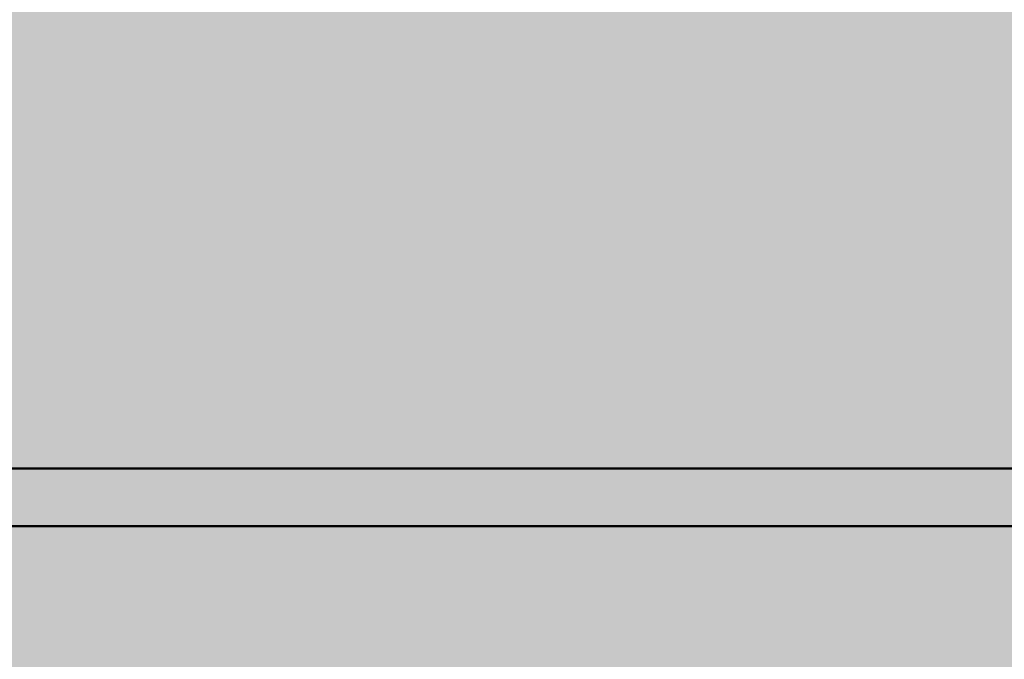
# Model space of a CAD drawing. Units: millimetres. Extents: x 0 to 2267, y 0 to 1823.
# Tile 136 of 256: x 1675 to 1760, y 1216 to 1271. Entities that reach past the tile are written whole.
import ezdxf

# ---------------------------------------------------------------- set-up
doc = ezdxf.new("R2010")
doc.units = ezdxf.units.MM
doc.header["$MEASUREMENT"] = 0
doc.layers.add('M-HATC', color=252, linetype='Continuous', lineweight=18)
doc.layers.add('M-OUTL', color=7, linetype='Continuous', lineweight=50)

msp = doc.modelspace()

# ---------------------------------------------------------------- hatches: boundary and pattern name
at = {"layer": 'M-HATC'}
h = msp.add_hatch(color=256, dxfattribs=at)
h.dxf.hatch_style = 1
h.paths.add_polyline_path([(2065.771, 1618.062, 0.236068), (2055.771, 1638.062), (1381.087, 1638.062, 0.236068), (1371.087, 1618.062), (1371.087, 1603.062), (2055.771, 1603.062), (2065.771, 1603.062)])
h.paths.add_polyline_path([(2062.772, 1550.296), (2062.772, 1560.296), (1374.086, 1560.296), (1374.086, 1550.296), (1374.086, 1540.296), (1384.086, 1540.296), (1389.086, 1540.296), (2062.772, 1540.296)])
h.paths.add_polyline_path([(1930.929, 1282.766), (1505.929, 1282.766), (1587.628, 1235.597, 0.131652), (1600.128, 1232.247), (1836.73, 1232.247, 0.131652), (1849.23, 1235.597)])
h.paths.add_polyline_path([(1930.929, 1117.417), (1905.929, 1117.417), (1505.929, 1117.417), (1505.929, 1077.417), (1930.929, 1077.417)])
h = msp.add_hatch(color=256, dxfattribs=at)
h.dxf.hatch_style = 1
h.paths.add_polyline_path([(2055.771, 1603.062), (1381.087, 1603.062), (1381.087, 1598.062), (2055.771, 1598.062)])
h.paths.add_polyline_path([(2055.771, 1598.062), (1381.087, 1598.062), (1381.087, 1593.062), (2055.771, 1593.062)])
h.paths.add_polyline_path([(2051.307, 1536.761), (1385.55, 1536.761), (1385.55, 1526.761), (1387.55, 1526.761), (1388.537, 1525.053), (1385.332, 1521.233), (1385.332, 1521.223), (2050.254, 1522.749), (2048.321, 1525.053), (2049.307, 1526.761), (2051.307, 1526.761)])
edge = h.paths.add_edge_path()
edge.add_arc((1847.535, 1379.149), 135, 222.60306, 222.89085, ccw=False)
edge.add_line((1748.166, 1287.766), (1683.092, 1287.766))
edge.add_arc((1583.724, 1379.149), 135, 317.10915, 317.39694, ccw=False)
edge.add_arc((1678.969, 1290.671), 5, 222.89085, 317.10915, ccw=False)
edge.add_arc((1774.213, 1379.149), 135, 222.60306, 222.89085, ccw=False)
edge.add_line((1674.845, 1287.766), (1609.771, 1287.766))
edge.add_arc((1510.403, 1379.149), 135, 317.10915, 317.39694, ccw=False)
edge.add_arc((1605.647, 1290.671), 5, 222.89085, 317.10915, ccw=False)
edge.add_arc((1700.892, 1379.149), 135, 222.60306, 222.89085, ccw=False)
edge.add_line((1601.524, 1287.766), (1536.45, 1287.766))
edge.add_arc((1437.081, 1379.149), 135, 317.10915, 317.39694, ccw=False)
edge.add_arc((1532.326, 1290.671), 5, 222.89085, 317.10915, ccw=False)
edge.add_arc((1627.571, 1379.149), 135, 222.60306, 222.89085, ccw=False)
edge.add_line((1528.203, 1287.766), (1505.929, 1287.766))
edge.add_spline(control_points=[(1505.929, 1287.766), (1504.262, 1287.766), (1504.262, 1282.766), (1505.929, 1282.766)], knot_values=[0, 0, 0, 0, 5, 5, 5, 5], degree=3, periodic=0)
edge.add_line((1505.929, 1282.766), (1930.929, 1282.766))
edge.add_spline(control_points=[(1930.929, 1282.766), (1932.596, 1282.766), (1932.596, 1287.766), (1930.929, 1287.766)], knot_values=[0, 0, 0, 0, 5, 5, 5, 5], degree=3, periodic=0)
edge.add_line((1930.929, 1287.766), (1903.056, 1287.766))
edge.add_arc((1803.688, 1379.149), 135, 317.10915, 317.39694, ccw=False)
edge.add_arc((1898.932, 1290.671), 5, 222.89085, 317.10915, ccw=False)
edge.add_arc((1994.177, 1379.149), 135, 222.60306, 222.89085, ccw=False)
edge.add_line((1894.809, 1287.766), (1829.735, 1287.766))
edge.add_arc((1730.366, 1379.149), 135, 317.10915, 317.39694, ccw=False)
edge.add_arc((1825.611, 1290.671), 5, 222.89085, 317.10915, ccw=False)
edge.add_arc((1920.856, 1379.149), 135, 222.60306, 222.89085, ccw=False)
edge.add_line((1821.487, 1287.766), (1756.413, 1287.766))
edge.add_arc((1657.045, 1379.149), 135, 317.10915, 317.39694, ccw=False)
edge.add_arc((1752.29, 1290.671), 5, 222.89085, 317.10915, ccw=False)
edge = h.paths.add_edge_path()
edge.add_spline(control_points=[(1843.429, 1227.247), (1845.096, 1227.247), (1845.096, 1232.247), (1843.429, 1232.247)], knot_values=[0, 0, 0, 0, 5, 5, 5, 5], degree=3, periodic=0)
edge.add_line((1843.429, 1232.247), (1593.429, 1232.247))
edge.add_spline(control_points=[(1593.429, 1232.247), (1591.762, 1232.247), (1591.762, 1227.247), (1593.429, 1227.247)], knot_values=[0, 0, 0, 0, 5, 5, 5, 5], degree=3, periodic=0)
edge.add_line((1593.429, 1227.247), (1843.429, 1227.247))
h.paths.add_polyline_path([(1905.929, 1127.417), (1530.929, 1127.417, 0.414214), (1520.929, 1117.417), (1530.929, 1117.417), (1915.929, 1117.417, 0.414214)])
edge = h.paths.add_edge_path()
edge.add_arc((1397.086, 1498.408), 12.73, 90.78215, 190.87871, ccw=False)
edge.add_line((1396.912, 1511.136), (1428.01, 1511.349))
edge.add_line((1428.01, 1511.349), (1433.01, 1511.349))
edge.add_line((1433.01, 1511.349), (1434.439, 1511.349))
edge.add_arc((1419.474, 1498.08), 20, 41.561, 74.08211)
edge.add_line((1424.959, 1517.314), (1399.935, 1517.256))
edge.add_spline(control_points=[(1399.931, 1517.256), (1399.884, 1517.213), (1399.833, 1517.169), (1399.777, 1517.124)], knot_values=[11.567499, 11.567499, 11.567499, 11.567499, 11.814249, 11.814249, 11.814249, 11.814249], degree=3, periodic=0)
edge.add_spline(control_points=[(1399.633, 1517.01), (1399.583, 1516.972), (1399.531, 1516.934), (1399.476, 1516.895)], knot_values=[11.167718, 11.167718, 11.167718, 11.167718, 11.365188, 11.365188, 11.365188, 11.365188], degree=3, periodic=0)
edge.add_spline(control_points=[(1399.34, 1516.8), (1399.151, 1516.672), (1398.938, 1516.538), (1398.704, 1516.399)], knot_values=[10.376405, 10.376405, 10.376405, 10.376405, 11.00994, 11.00994, 11.00994, 11.00994], degree=3, periodic=0)
edge.add_spline(control_points=[(1398.657, 1516.372), (1398.579, 1516.326), (1398.498, 1516.28), (1398.415, 1516.233)], knot_values=[10.125175, 10.125175, 10.125175, 10.125175, 10.334406, 10.334406, 10.334406, 10.334406], degree=3, periodic=0)
edge.add_spline(control_points=[(1398.264, 1516.149), (1398.196, 1516.111), (1398.126, 1516.073), (1398.055, 1516.035)], knot_values=[9.832246, 9.832246, 9.832246, 9.832246, 9.999658, 9.999658, 9.999658, 9.999658], degree=3, periodic=0)
edge.add_spline(control_points=[(1397.999, 1516.005), (1397.731, 1515.862), (1397.446, 1515.717), (1397.147, 1515.571)], knot_values=[9.161808, 9.161808, 9.161808, 9.161808, 9.787769, 9.787769, 9.787769, 9.787769], degree=3, periodic=0)
edge.add_spline(control_points=[(1397.147, 1515.571), (1396.842, 1515.423), (1396.522, 1515.274), (1396.191, 1515.126)], knot_values=[8.524455, 8.524455, 8.524455, 8.524455, 9.161808, 9.161808, 9.161808, 9.161808], degree=3, periodic=0)
edge.add_spline(control_points=[(1396.078, 1515.076), (1395.985, 1515.035), (1395.892, 1514.994), (1395.798, 1514.953)], knot_values=[8.275193, 8.275193, 8.275193, 8.275193, 8.451726, 8.451726, 8.451726, 8.451726], degree=3, periodic=0)
edge.add_spline(control_points=[(1395.602, 1514.869), (1395.5, 1514.826), (1395.397, 1514.782), (1395.293, 1514.739)], knot_values=[7.962917, 7.962917, 7.962917, 7.962917, 8.152764, 8.152764, 8.152764, 8.152764], degree=3, periodic=0)
edge.add_spline(control_points=[(1395.212, 1514.706), (1394.828, 1514.547), (1394.435, 1514.393), (1394.036, 1514.244)], knot_values=[7.21254, 7.21254, 7.21254, 7.21254, 7.913148, 7.913148, 7.913148, 7.913148], degree=3, periodic=0)
edge.add_spline(control_points=[(1394.036, 1514.244), (1393.708, 1514.121), (1393.375, 1514.003), (1393.043, 1513.889)], knot_values=[6.633733, 6.633733, 6.633733, 6.633733, 7.21254, 7.21254, 7.21254, 7.21254], degree=3, periodic=0)
edge.add_spline(control_points=[(1392.821, 1513.815), (1392.72, 1513.781), (1392.618, 1513.748), (1392.517, 1513.715)], knot_values=[6.328796, 6.328796, 6.328796, 6.328796, 6.505493, 6.505493, 6.505493, 6.505493], degree=3, periodic=0)
edge.add_spline(control_points=[(1392.517, 1513.715), (1392.319, 1513.652), (1392.121, 1513.59), (1391.924, 1513.531)], knot_values=[5.984605, 5.984605, 5.984605, 5.984605, 6.328796, 6.328796, 6.328796, 6.328796], degree=3, periodic=0)
edge.add_spline(control_points=[(1391.792, 1513.491), (1391.312, 1513.35), (1390.838, 1513.224), (1390.378, 1513.117)], knot_values=[5.066697, 5.066697, 5.066697, 5.066697, 5.907055, 5.907055, 5.907055, 5.907055], degree=3, periodic=0)
edge.add_spline(control_points=[(1390.378, 1513.117), (1390.18, 1513.071), (1389.984, 1513.028), (1389.791, 1512.99)], knot_values=[4.70367, 4.70367, 4.70367, 4.70367, 5.066695, 5.066695, 5.066695, 5.066695], degree=3, periodic=0)
edge.add_spline(control_points=[(1389.422, 1512.92), (1389.246, 1512.889), (1389.073, 1512.862), (1388.904, 1512.838)], knot_values=[4.130571, 4.130571, 4.130571, 4.130571, 4.469816, 4.469816, 4.469816, 4.469816], degree=3, periodic=0)
edge.add_spline(control_points=[(1388.904, 1512.838), (1388.591, 1512.795), (1388.291, 1512.764), (1388.007, 1512.749)], knot_values=[3.504031, 3.504031, 3.504031, 3.504031, 4.130571, 4.130571, 4.130571, 4.130571], degree=3, periodic=0)
edge.add_spline(control_points=[(1387.936, 1512.746), (1387.854, 1512.742), (1387.773, 1512.74), (1387.694, 1512.739)], knot_values=[3.268866, 3.268866, 3.268866, 3.268866, 3.451164, 3.451164, 3.451164, 3.451164], degree=3, periodic=0)
edge.add_spline(control_points=[(1387.335, 1512.744), (1387.208, 1512.75), (1387.085, 1512.76), (1386.967, 1512.774)], knot_values=[2.670686, 2.670686, 2.670686, 2.670686, 2.984, 2.984, 2.984, 2.984], degree=3, periodic=0)
edge.add_spline(control_points=[(1386.833, 1512.792), (1386.821, 1512.794), (1386.809, 1512.796), (1386.797, 1512.798)], knot_values=[2.516981, 2.516981, 2.516981, 2.516981, 2.549528, 2.549528, 2.549528, 2.549528], degree=3, periodic=0)
edge.add_spline(control_points=[(1386.453, 1512.873), (1386.426, 1512.881), (1386.399, 1512.889), (1386.373, 1512.897)], knot_values=[2.095869, 2.095869, 2.095869, 2.095869, 2.17941, 2.17941, 2.17941, 2.17941], degree=3, periodic=0)
edge.add_spline(control_points=[(1386.069, 1513.019), (1386.063, 1513.022), (1386.058, 1513.025), (1386.052, 1513.028)], knot_values=[1.72453, 1.72453, 1.72453, 1.72453, 1.745933, 1.745933, 1.745933, 1.745933], degree=3, periodic=0)
edge.add_arc((1399.474, 1498.08), 20, 131.82432, 180)
edge.add_arc((1630.334, 1505.548), 250.971, 181.70518, 236.42798)
edge.add_arc((1605.34, 1483.304), 218.782, 238.66083, 243.34961)
edge.add_arc((1647.091, 1510.359), 262.899, 183.12984, 237.85344, ccw=False)
h.paths.add_polyline_path([(1406.537, 1391.964, 0.149382), (1491.551, 1296.442, -0.129517)], flags=17)
edge = h.paths.add_edge_path()
edge.add_arc((2037.384, 1498.08), 20, 0, 48.26587)
edge.add_spline(control_points=[(2050.697, 1513.005), (2050.651, 1512.985), (2050.603, 1512.966), (2050.554, 1512.948)], knot_values=[1.835652, 1.835652, 1.835652, 1.835652, 2.000781, 2.000781, 2.000781, 2.000781], degree=3, periodic=0)
edge.add_spline(control_points=[(2050.462, 1512.917), (2050.479, 1512.922), (2050.496, 1512.928), (2050.513, 1512.934)], knot_values=[2.045477, 2.045477, 2.045477, 2.045477, 2.101389, 2.101389, 2.101389, 2.101389], degree=3, periodic=0)
edge.add_spline(control_points=[(2050.129, 1512.834), (2050.198, 1512.847), (2050.266, 1512.862), (2050.331, 1512.879)], knot_values=[2.237629, 2.237629, 2.237629, 2.237629, 2.435841, 2.435841, 2.435841, 2.435841], degree=3, periodic=0)
edge.add_spline(control_points=[(2050.095, 1512.828), (2050.106, 1512.83), (2050.118, 1512.832), (2050.129, 1512.834)], knot_values=[2.435841, 2.435841, 2.435841, 2.435841, 2.468321, 2.468321, 2.468321, 2.468321], degree=3, periodic=0)
edge.add_spline(control_points=[(2049.784, 1512.785), (2049.855, 1512.792), (2049.924, 1512.801), (2049.992, 1512.811)], knot_values=[2.563852, 2.563852, 2.563852, 2.563852, 2.748541, 2.748541, 2.748541, 2.748541], degree=3, periodic=0)
edge.add_spline(control_points=[(2049.405, 1512.762), (2049.536, 1512.765), (2049.663, 1512.773), (2049.784, 1512.785)], knot_values=[2.748541, 2.748541, 2.748541, 2.748541, 3.064882, 3.064882, 3.064882, 3.064882], degree=3, periodic=0)
edge.add_spline(control_points=[(2049.17, 1512.76), (2049.234, 1512.759), (2049.297, 1512.759), (2049.358, 1512.761)], knot_values=[3.102309, 3.102309, 3.102309, 3.102309, 3.2503, 3.2503, 3.2503, 3.2503], degree=3, periodic=0)
edge.add_spline(control_points=[(2048.857, 1512.769), (2048.964, 1512.764), (2049.068, 1512.761), (2049.17, 1512.76)], knot_values=[3.2503, 3.2503, 3.2503, 3.2503, 3.486069, 3.486069, 3.486069, 3.486069], degree=3, periodic=0)
edge.add_spline(control_points=[(2048.692, 1512.779), (2048.373, 1512.801), (2048.035, 1512.841), (2047.682, 1512.897)], knot_values=[3.606429, 3.606429, 3.606429, 3.606429, 4.2989, 4.2989, 4.2989, 4.2989], degree=3, periodic=0)
edge.add_spline(control_points=[(2047.682, 1512.897), (2047.546, 1512.919), (2047.408, 1512.942), (2047.268, 1512.969)], knot_values=[4.2989, 4.2989, 4.2989, 4.2989, 4.565769, 4.565769, 4.565769, 4.565769], degree=3, periodic=0)
edge.add_spline(control_points=[(2047.268, 1512.969), (2047.145, 1512.991), (2047.021, 1513.016), (2046.895, 1513.042)], knot_values=[4.565769, 4.565769, 4.565769, 4.565769, 4.799971, 4.799971, 4.799971, 4.799971], degree=3, periodic=0)
edge.add_spline(control_points=[(2046.895, 1513.042), (2046.529, 1513.119), (2046.151, 1513.209), (2045.768, 1513.311)], knot_values=[4.799971, 4.799971, 4.799971, 4.799971, 5.483718, 5.483718, 5.483718, 5.483718], degree=3, periodic=0)
edge.add_spline(control_points=[(2045.768, 1513.311), (2045.372, 1513.415), (2044.97, 1513.532), (2044.566, 1513.659)], knot_values=[5.483718, 5.483718, 5.483718, 5.483718, 6.187866, 6.187866, 6.187866, 6.187866], degree=3, periodic=0)
edge.add_spline(control_points=[(2044.566, 1513.659), (2044.415, 1513.706), (2044.263, 1513.755), (2044.112, 1513.805)], knot_values=[6.187866, 6.187866, 6.187866, 6.187866, 6.451551, 6.451551, 6.451551, 6.451551], degree=3, periodic=0)
edge.add_spline(control_points=[(2044.112, 1513.805), (2043.997, 1513.843), (2043.882, 1513.881), (2043.767, 1513.92)], knot_values=[6.451551, 6.451551, 6.451551, 6.451551, 6.651434, 6.651434, 6.651434, 6.651434], degree=3, periodic=0)
edge.add_spline(control_points=[(2043.767, 1513.92), (2043.372, 1514.055), (2042.977, 1514.198), (2042.589, 1514.346)], knot_values=[6.651434, 6.651434, 6.651434, 6.651434, 7.338879, 7.338879, 7.338879, 7.338879], degree=3, periodic=0)
edge.add_spline(control_points=[(2042.589, 1514.346), (2042.164, 1514.507), (2041.746, 1514.675), (2041.341, 1514.846)], knot_values=[7.338879, 7.338879, 7.338879, 7.338879, 8.089209, 8.089209, 8.089209, 8.089209], degree=3, periodic=0)
edge.add_spline(control_points=[(2041.341, 1514.846), (2041.103, 1514.946), (2040.869, 1515.048), (2040.64, 1515.15)], knot_values=[8.089209, 8.089209, 8.089209, 8.089209, 8.529587, 8.529587, 8.529587, 8.529587], degree=3, periodic=0)
edge.add_spline(control_points=[(2040.51, 1515.209), (2040.082, 1515.402), (2039.675, 1515.597), (2039.295, 1515.789)], knot_values=[8.613818, 8.613818, 8.613818, 8.613818, 9.44571, 9.44571, 9.44571, 9.44571], degree=3, periodic=0)
edge.add_spline(control_points=[(2039.295, 1515.789), (2039.062, 1515.907), (2038.839, 1516.025), (2038.629, 1516.14)], knot_values=[9.44571, 9.44571, 9.44571, 9.44571, 9.956404, 9.956404, 9.956404, 9.956404], degree=3, periodic=0)
edge.add_spline(control_points=[(2038.629, 1516.14), (2038.519, 1516.2), (2038.412, 1516.26), (2038.309, 1516.319)], knot_values=[9.956404, 9.956404, 9.956404, 9.956404, 10.223542, 10.223542, 10.223542, 10.223542], degree=3, periodic=0)
edge.add_spline(control_points=[(2038.309, 1516.319), (2038.214, 1516.374), (2038.122, 1516.428), (2038.033, 1516.481)], knot_values=[10.223542, 10.223542, 10.223542, 10.223542, 10.47051, 10.47051, 10.47051, 10.47051], degree=3, periodic=0)
edge.add_spline(control_points=[(2038.033, 1516.481), (2037.786, 1516.63), (2037.564, 1516.773), (2037.372, 1516.909)], knot_values=[10.47051, 10.47051, 10.47051, 10.47051, 11.15767, 11.15767, 11.15767, 11.15767], degree=3, periodic=0)
edge.add_spline(control_points=[(2037.372, 1516.909), (2037.279, 1516.975), (2037.193, 1517.04), (2037.114, 1517.102)], knot_values=[11.15767, 11.15767, 11.15767, 11.15767, 11.49227, 11.49227, 11.49227, 11.49227], degree=3, periodic=0)
edge.add_spline(control_points=[(2036.856, 1517.326), (2036.915, 1517.269), (2036.981, 1517.21), (2037.056, 1517.149)], knot_values=[11.577341, 11.577341, 11.577341, 11.577341, 11.91035, 11.91035, 11.91035, 11.91035], degree=3, periodic=0)
edge.add_spline(control_points=[(2036.807, 1517.375), (2036.823, 1517.359), (2036.839, 1517.342), (2036.856, 1517.326)], knot_values=[11.91035, 11.91035, 11.91035, 11.91035, 12.007402, 12.007402, 12.007402, 12.007402], degree=3, periodic=0)
edge.add_spline(control_points=[(2036.702, 1517.494), (2036.71, 1517.483), (2036.72, 1517.472), (2036.729, 1517.461)], knot_values=[12.184155, 12.184155, 12.184155, 12.184155, 12.255409, 12.255409, 12.255409, 12.255409], degree=3, periodic=0)
edge.add_spline(control_points=[(2036.616, 1517.621), (2036.62, 1517.613), (2036.624, 1517.606), (2036.629, 1517.598)], knot_values=[12.487913, 12.487913, 12.487913, 12.487913, 12.541035, 12.541035, 12.541035, 12.541035], degree=3, periodic=0)
edge.add_spline(control_points=[(2036.563, 1517.786), (2036.564, 1517.779), (2036.564, 1517.773), (2036.565, 1517.766)], knot_values=[12.911761, 12.911761, 12.911761, 12.911761, 12.968286, 12.968286, 12.968286, 12.968286], degree=3, periodic=0)
edge.add_spline(control_points=[(2036.617, 1517.93), (2036.612, 1517.926), (2036.609, 1517.921), (2036.605, 1517.916)], knot_values=[13.382527, 13.382527, 13.382527, 13.382527, 13.433791, 13.433791, 13.433791, 13.433791], degree=3, periodic=0)
edge.add_spline(control_points=[(2036.749, 1518.017), (2036.736, 1518.012), (2036.724, 1518.006), (2036.712, 1518)], knot_values=[13.726299, 13.726299, 13.726299, 13.726299, 13.809928, 13.809928, 13.809928, 13.809928], degree=3, periodic=0)
edge.add_spline(control_points=[(2036.86, 1518.053), (2036.839, 1518.047), (2036.818, 1518.042), (2036.799, 1518.035)], knot_values=[13.910887, 13.910887, 13.910887, 13.910887, 14.02153, 14.02153, 14.02153, 14.02153], degree=3, periodic=0)
edge.add_line((2036.964, 1518.08), (2032.384, 1518.08))
edge.add_line((2032.384, 1518.08), (2027.384, 1518.08))
edge.add_line((2027.384, 1518.08), (2022.384, 1518.08))
edge.add_line((2022.384, 1518.08), (2017.384, 1518.08))
edge.add_arc((2017.384, 1498.08), 20, 90, 138.439)
edge.add_line((2002.419, 1511.349), (2003.848, 1511.349))
edge.add_line((2003.848, 1511.349), (2008.848, 1511.349))
edge.add_line((2008.848, 1511.349), (2039.772, 1511.138))
edge.add_arc((2039.772, 1498.408), 12.73, -10.87871, 90, ccw=False)
edge.add_arc((1789.767, 1510.359), 262.899, 302.14656, 356.87016, ccw=False)
edge.add_arc((1831.518, 1483.304), 218.782, 296.65039, 301.33917)
edge.add_arc((1806.524, 1505.548), 250.971, 303.57202, 358.29482)
h.paths.add_polyline_path([(2030.321, 1391.964, -0.129517), (1945.307, 1296.442, 0.149382)], flags=17)
edge = h.paths.add_edge_path()
edge.add_spline(control_points=[(2037.246, 1518.082), (2037.29, 1518.081), (2037.336, 1518.08), (2037.384, 1518.08)], knot_values=[0.000012, 0.000012, 0.000012, 0.000012, 0.144754, 0.144754, 0.144754, 0.144754], degree=3, periodic=0)
edge.add_line((2037.336, 1518.08), (2037.01, 1518.08))
edge.add_spline(control_points=[(2037.01, 1518.08), (2036.982, 1518.077), (2036.956, 1518.073), (2036.931, 1518.068)], knot_values=[14.13465, 14.13465, 14.13465, 14.13465, 14.247197, 14.247197, 14.247197, 14.247197], degree=3, periodic=0)
edge.add_spline(control_points=[(2036.931, 1518.068), (2036.928, 1518.067), (2036.924, 1518.067), (2036.921, 1518.066)], knot_values=[14.118315, 14.118315, 14.118315, 14.118315, 14.13465, 14.13465, 14.13465, 14.13465], degree=3, periodic=0)
edge.add_spline(control_points=[(2036.921, 1518.066), (2036.912, 1518.064), (2036.903, 1518.063), (2036.895, 1518.061)], knot_values=[14.078086, 14.078086, 14.078086, 14.078086, 14.118315, 14.118315, 14.118315, 14.118315], degree=3, periodic=0)
edge.add_spline(control_points=[(2036.895, 1518.061), (2036.883, 1518.058), (2036.872, 1518.056), (2036.86, 1518.053)], knot_values=[14.02153, 14.02153, 14.02153, 14.02153, 14.078086, 14.078086, 14.078086, 14.078086], degree=3, periodic=0)
edge.add_spline(control_points=[(2036.86, 1518.053), (2036.839, 1518.047), (2036.818, 1518.042), (2036.799, 1518.035)], knot_values=[13.910887, 13.910887, 13.910887, 13.910887, 14.02153, 14.02153, 14.02153, 14.02153], degree=3, periodic=0)
edge.add_spline(control_points=[(2036.799, 1518.035), (2036.798, 1518.035), (2036.797, 1518.035), (2036.797, 1518.035)], knot_values=[13.906906, 13.906906, 13.906906, 13.906906, 13.910887, 13.910887, 13.910887, 13.910887], degree=3, periodic=0)
edge.add_spline(control_points=[(2036.797, 1518.035), (2036.788, 1518.032), (2036.78, 1518.029), (2036.772, 1518.026)], knot_values=[13.857826, 13.857826, 13.857826, 13.857826, 13.906906, 13.906906, 13.906906, 13.906906], degree=3, periodic=0)
edge.add_spline(control_points=[(2036.772, 1518.026), (2036.764, 1518.023), (2036.756, 1518.02), (2036.749, 1518.017)], knot_values=[13.809928, 13.809928, 13.809928, 13.809928, 13.857826, 13.857826, 13.857826, 13.857826], degree=3, periodic=0)
edge.add_spline(control_points=[(2036.749, 1518.017), (2036.736, 1518.012), (2036.724, 1518.006), (2036.712, 1518)], knot_values=[13.726299, 13.726299, 13.726299, 13.726299, 13.809928, 13.809928, 13.809928, 13.809928], degree=3, periodic=0)
edge.add_spline(control_points=[(2036.712, 1518), (2036.712, 1518), (2036.712, 1518), (2036.711, 1518)], knot_values=[13.723993, 13.723993, 13.723993, 13.723993, 13.726299, 13.726299, 13.726299, 13.726299], degree=3, periodic=0)
edge.add_spline(control_points=[(2036.711, 1518), (2036.706, 1517.997), (2036.701, 1517.994), (2036.696, 1517.992)], knot_values=[13.686536, 13.686536, 13.686536, 13.686536, 13.723993, 13.723993, 13.723993, 13.723993], degree=3, periodic=0)
edge.add_spline(control_points=[(2036.696, 1517.992), (2036.692, 1517.989), (2036.687, 1517.987), (2036.683, 1517.984)], knot_values=[13.651251, 13.651251, 13.651251, 13.651251, 13.686536, 13.686536, 13.686536, 13.686536], degree=3, periodic=0)
edge.add_spline(control_points=[(2036.683, 1517.984), (2036.676, 1517.98), (2036.67, 1517.976), (2036.664, 1517.971)], knot_values=[13.596804, 13.596804, 13.596804, 13.596804, 13.651251, 13.651251, 13.651251, 13.651251], degree=3, periodic=0)
edge.add_spline(control_points=[(2036.664, 1517.971), (2036.664, 1517.971), (2036.663, 1517.971), (2036.663, 1517.971)], knot_values=[13.593956, 13.593956, 13.593956, 13.593956, 13.596804, 13.596804, 13.596804, 13.596804], degree=3, periodic=0)
edge.add_spline(control_points=[(2036.663, 1517.971), (2036.66, 1517.969), (2036.658, 1517.967), (2036.655, 1517.965)], knot_values=[13.570322, 13.570322, 13.570322, 13.570322, 13.593956, 13.593956, 13.593956, 13.593956], degree=3, periodic=0)
edge.add_spline(control_points=[(2036.655, 1517.965), (2036.653, 1517.963), (2036.65, 1517.961), (2036.647, 1517.959)], knot_values=[13.545477, 13.545477, 13.545477, 13.545477, 13.570322, 13.570322, 13.570322, 13.570322], degree=3, periodic=0)
edge.add_spline(control_points=[(2036.647, 1517.959), (2036.647, 1517.959), (2036.647, 1517.959), (2036.647, 1517.959)], knot_values=[13.543931, 13.543931, 13.543931, 13.543931, 13.545477, 13.545477, 13.545477, 13.545477], degree=3, periodic=0)
edge.add_spline(control_points=[(2036.647, 1517.959), (2036.641, 1517.954), (2036.636, 1517.949), (2036.631, 1517.945)], knot_values=[13.488237, 13.488237, 13.488237, 13.488237, 13.543931, 13.543931, 13.543931, 13.543931], degree=3, periodic=0)
edge.add_spline(control_points=[(2036.631, 1517.945), (2036.628, 1517.942), (2036.626, 1517.94), (2036.623, 1517.937)], knot_values=[13.460307, 13.460307, 13.460307, 13.460307, 13.488237, 13.488237, 13.488237, 13.488237], degree=3, periodic=0)
edge.add_spline(control_points=[(2036.623, 1517.937), (2036.622, 1517.936), (2036.62, 1517.934), (2036.618, 1517.932)], knot_values=[13.439712, 13.439712, 13.439712, 13.439712, 13.460307, 13.460307, 13.460307, 13.460307], degree=3, periodic=0)
edge.add_spline(control_points=[(2036.618, 1517.932), (2036.618, 1517.931), (2036.617, 1517.931), (2036.617, 1517.93)], knot_values=[13.433791, 13.433791, 13.433791, 13.433791, 13.439712, 13.439712, 13.439712, 13.439712], degree=3, periodic=0)
edge.add_spline(control_points=[(2036.617, 1517.93), (2036.612, 1517.926), (2036.609, 1517.921), (2036.605, 1517.916)], knot_values=[13.382527, 13.382527, 13.382527, 13.382527, 13.433791, 13.433791, 13.433791, 13.433791], degree=3, periodic=0)
edge.add_spline(control_points=[(2036.605, 1517.916), (2036.603, 1517.913), (2036.6, 1517.91), (2036.598, 1517.907)], knot_values=[13.350017, 13.350017, 13.350017, 13.350017, 13.382527, 13.382527, 13.382527, 13.382527], degree=3, periodic=0)
edge.add_spline(control_points=[(2036.598, 1517.907), (2036.597, 1517.906), (2036.596, 1517.904), (2036.595, 1517.903)], knot_values=[13.333922, 13.333922, 13.333922, 13.333922, 13.350017, 13.350017, 13.350017, 13.350017], degree=3, periodic=0)
edge.add_spline(control_points=[(2036.595, 1517.903), (2036.595, 1517.902), (2036.594, 1517.901), (2036.593, 1517.9)], knot_values=[13.323828, 13.323828, 13.323828, 13.323828, 13.333922, 13.333922, 13.333922, 13.333922], degree=3, periodic=0)
edge.add_spline(control_points=[(2036.593, 1517.9), (2036.59, 1517.895), (2036.588, 1517.891), (2036.585, 1517.886)], knot_values=[13.277545, 13.277545, 13.277545, 13.277545, 13.323828, 13.323828, 13.323828, 13.323828], degree=3, periodic=0)
edge.add_spline(control_points=[(2036.585, 1517.886), (2036.584, 1517.883), (2036.582, 1517.879), (2036.58, 1517.875)], knot_values=[13.240119, 13.240119, 13.240119, 13.240119, 13.277545, 13.277545, 13.277545, 13.277545], degree=3, periodic=0)
edge.add_spline(control_points=[(2036.58, 1517.875), (2036.58, 1517.874), (2036.579, 1517.873), (2036.578, 1517.872)], knot_values=[13.228211, 13.228211, 13.228211, 13.228211, 13.240119, 13.240119, 13.240119, 13.240119], degree=3, periodic=0)
edge.add_spline(control_points=[(2036.578, 1517.872), (2036.578, 1517.87), (2036.577, 1517.869), (2036.577, 1517.868)], knot_values=[13.215717, 13.215717, 13.215717, 13.215717, 13.228211, 13.228211, 13.228211, 13.228211], degree=3, periodic=0)
edge.add_spline(control_points=[(2036.577, 1517.868), (2036.575, 1517.864), (2036.574, 1517.86), (2036.573, 1517.857)], knot_values=[13.179847, 13.179847, 13.179847, 13.179847, 13.215717, 13.215717, 13.215717, 13.215717], degree=3, periodic=0)
edge.add_spline(control_points=[(2036.573, 1517.857), (2036.571, 1517.851), (2036.57, 1517.846), (2036.569, 1517.841)], knot_values=[13.132017, 13.132017, 13.132017, 13.132017, 13.179847, 13.179847, 13.179847, 13.179847], degree=3, periodic=0)
edge.add_spline(control_points=[(2036.569, 1517.841), (2036.568, 1517.84), (2036.568, 1517.839), (2036.568, 1517.838)], knot_values=[13.122482, 13.122482, 13.122482, 13.122482, 13.132017, 13.132017, 13.132017, 13.132017], degree=3, periodic=0)
edge.add_spline(control_points=[(2036.568, 1517.838), (2036.568, 1517.836), (2036.567, 1517.835), (2036.567, 1517.833)], knot_values=[13.105592, 13.105592, 13.105592, 13.105592, 13.122482, 13.122482, 13.122482, 13.122482], degree=3, periodic=0)
edge.add_spline(control_points=[(2036.567, 1517.833), (2036.566, 1517.829), (2036.566, 1517.826), (2036.565, 1517.822)], knot_values=[13.074063, 13.074063, 13.074063, 13.074063, 13.105592, 13.105592, 13.105592, 13.105592], degree=3, periodic=0)
edge.add_spline(control_points=[(2036.565, 1517.822), (2036.565, 1517.822), (2036.565, 1517.822), (2036.565, 1517.822)], knot_values=[13.074043, 13.074043, 13.074043, 13.074043, 13.074063, 13.074063, 13.074063, 13.074063], degree=3, periodic=0)
edge.add_spline(control_points=[(2036.565, 1517.822), (2036.564, 1517.816), (2036.564, 1517.811), (2036.564, 1517.805)], knot_values=[13.021884, 13.021884, 13.021884, 13.021884, 13.074043, 13.074043, 13.074043, 13.074043], degree=3, periodic=0)
edge.add_spline(control_points=[(2036.564, 1517.805), (2036.564, 1517.804), (2036.564, 1517.803), (2036.564, 1517.803)], knot_values=[13.01674, 13.01674, 13.01674, 13.01674, 13.021884, 13.021884, 13.021884, 13.021884], degree=3, periodic=0)
edge.add_spline(control_points=[(2036.564, 1517.803), (2036.563, 1517.801), (2036.563, 1517.798), (2036.563, 1517.796)], knot_values=[12.996438, 12.996438, 12.996438, 12.996438, 13.01674, 13.01674, 13.01674, 13.01674], degree=3, periodic=0)
edge.add_spline(control_points=[(2036.563, 1517.796), (2036.563, 1517.793), (2036.563, 1517.789), (2036.563, 1517.786)], knot_values=[12.968286, 12.968286, 12.968286, 12.968286, 12.996438, 12.996438, 12.996438, 12.996438], degree=3, periodic=0)
edge.add_spline(control_points=[(2036.563, 1517.786), (2036.564, 1517.779), (2036.564, 1517.773), (2036.565, 1517.766)], knot_values=[12.911761, 12.911761, 12.911761, 12.911761, 12.968286, 12.968286, 12.968286, 12.968286], degree=3, periodic=0)
edge.add_spline(control_points=[(2036.565, 1517.766), (2036.565, 1517.766), (2036.565, 1517.766), (2036.565, 1517.766)], knot_values=[12.911017, 12.911017, 12.911017, 12.911017, 12.911761, 12.911761, 12.911761, 12.911761], degree=3, periodic=0)
edge.add_spline(control_points=[(2036.565, 1517.766), (2036.565, 1517.762), (2036.566, 1517.759), (2036.566, 1517.756)], knot_values=[12.88528, 12.88528, 12.88528, 12.88528, 12.911017, 12.911017, 12.911017, 12.911017], degree=3, periodic=0)
edge.add_spline(control_points=[(2036.566, 1517.756), (2036.567, 1517.753), (2036.567, 1517.751), (2036.568, 1517.748)], knot_values=[12.862519, 12.862519, 12.862519, 12.862519, 12.88528, 12.88528, 12.88528, 12.88528], degree=3, periodic=0)
edge.add_spline(control_points=[(2036.568, 1517.748), (2036.568, 1517.747), (2036.568, 1517.747), (2036.568, 1517.746)], knot_values=[12.858885, 12.858885, 12.858885, 12.858885, 12.862519, 12.862519, 12.862519, 12.862519], degree=3, periodic=0)
edge.add_spline(control_points=[(2036.568, 1517.746), (2036.569, 1517.74), (2036.571, 1517.733), (2036.572, 1517.726)], knot_values=[12.8053, 12.8053, 12.8053, 12.8053, 12.858885, 12.858885, 12.858885, 12.858885], degree=3, periodic=0)
edge.add_spline(control_points=[(2036.572, 1517.726), (2036.573, 1517.723), (2036.574, 1517.719), (2036.576, 1517.715)], knot_values=[12.775176, 12.775176, 12.775176, 12.775176, 12.8053, 12.8053, 12.8053, 12.8053], degree=3, periodic=0)
edge.add_spline(control_points=[(2036.576, 1517.715), (2036.576, 1517.713), (2036.577, 1517.71), (2036.578, 1517.708)], knot_values=[12.756759, 12.756759, 12.756759, 12.756759, 12.775176, 12.775176, 12.775176, 12.775176], degree=3, periodic=0)
edge.add_spline(control_points=[(2036.578, 1517.708), (2036.578, 1517.707), (2036.578, 1517.706), (2036.579, 1517.705)], knot_values=[12.748742, 12.748742, 12.748742, 12.748742, 12.756759, 12.756759, 12.756759, 12.756759], degree=3, periodic=0)
edge.add_spline(control_points=[(2036.579, 1517.705), (2036.581, 1517.698), (2036.583, 1517.692), (2036.586, 1517.685)], knot_values=[12.69959, 12.69959, 12.69959, 12.69959, 12.748742, 12.748742, 12.748742, 12.748742], degree=3, periodic=0)
edge.add_spline(control_points=[(2036.586, 1517.685), (2036.588, 1517.68), (2036.59, 1517.675), (2036.592, 1517.669)], knot_values=[12.659038, 12.659038, 12.659038, 12.659038, 12.69959, 12.69959, 12.69959, 12.69959], degree=3, periodic=0)
edge.add_spline(control_points=[(2036.592, 1517.669), (2036.594, 1517.665), (2036.596, 1517.66), (2036.598, 1517.656)], knot_values=[12.626806, 12.626806, 12.626806, 12.626806, 12.659038, 12.659038, 12.659038, 12.659038], degree=3, periodic=0)
edge.add_spline(control_points=[(2036.598, 1517.656), (2036.598, 1517.655), (2036.599, 1517.654), (2036.599, 1517.653)], knot_values=[12.619394, 12.619394, 12.619394, 12.619394, 12.626806, 12.626806, 12.626806, 12.626806], degree=3, periodic=0)
edge.add_spline(control_points=[(2036.599, 1517.653), (2036.604, 1517.642), (2036.61, 1517.632), (2036.616, 1517.621)], knot_values=[12.541039, 12.541039, 12.541039, 12.541039, 12.619394, 12.619394, 12.619394, 12.619394], degree=3, periodic=0)
edge.add_spline(control_points=[(2036.616, 1517.621), (2036.616, 1517.621), (2036.616, 1517.621), (2036.616, 1517.621)], knot_values=[12.541035, 12.541035, 12.541035, 12.541035, 12.541039, 12.541039, 12.541039, 12.541039], degree=3, periodic=0)
edge.add_spline(control_points=[(2036.616, 1517.621), (2036.62, 1517.613), (2036.624, 1517.606), (2036.629, 1517.598)], knot_values=[12.487913, 12.487913, 12.487913, 12.487913, 12.541035, 12.541035, 12.541035, 12.541035], degree=3, periodic=0)
edge.add_spline(control_points=[(2036.629, 1517.598), (2036.633, 1517.592), (2036.637, 1517.585), (2036.641, 1517.579)], knot_values=[12.443982, 12.443982, 12.443982, 12.443982, 12.487913, 12.487913, 12.487913, 12.487913], degree=3, periodic=0)
edge.add_spline(control_points=[(2036.641, 1517.579), (2036.641, 1517.578), (2036.642, 1517.576), (2036.643, 1517.575)], knot_values=[12.434996, 12.434996, 12.434996, 12.434996, 12.443982, 12.443982, 12.443982, 12.443982], degree=3, periodic=0)
edge.add_spline(control_points=[(2036.643, 1517.575), (2036.653, 1517.56), (2036.664, 1517.544), (2036.676, 1517.528)], knot_values=[12.329647, 12.329647, 12.329647, 12.329647, 12.434996, 12.434996, 12.434996, 12.434996], degree=3, periodic=0)
edge.add_spline(control_points=[(2036.676, 1517.528), (2036.684, 1517.517), (2036.693, 1517.505), (2036.702, 1517.494)], knot_values=[12.255409, 12.255409, 12.255409, 12.255409, 12.329647, 12.329647, 12.329647, 12.329647], degree=3, periodic=0)
edge.add_spline(control_points=[(2036.702, 1517.494), (2036.71, 1517.483), (2036.72, 1517.472), (2036.729, 1517.461)], knot_values=[12.184155, 12.184155, 12.184155, 12.184155, 12.255409, 12.255409, 12.255409, 12.255409], degree=3, periodic=0)
edge.add_spline(control_points=[(2036.729, 1517.461), (2036.744, 1517.444), (2036.759, 1517.426), (2036.775, 1517.409)], knot_values=[12.075961, 12.075961, 12.075961, 12.075961, 12.184155, 12.184155, 12.184155, 12.184155], degree=3, periodic=0)
edge.add_spline(control_points=[(2036.775, 1517.409), (2036.776, 1517.407), (2036.777, 1517.406), (2036.778, 1517.405)], knot_values=[12.069502, 12.069502, 12.069502, 12.069502, 12.075961, 12.075961, 12.075961, 12.075961], degree=3, periodic=0)
edge.add_spline(control_points=[(2036.778, 1517.405), (2036.788, 1517.395), (2036.797, 1517.385), (2036.807, 1517.375)], knot_values=[12.007402, 12.007402, 12.007402, 12.007402, 12.069502, 12.069502, 12.069502, 12.069502], degree=3, periodic=0)
edge.add_spline(control_points=[(2036.807, 1517.375), (2036.823, 1517.359), (2036.839, 1517.342), (2036.856, 1517.326)], knot_values=[11.91035, 11.91035, 11.91035, 11.91035, 12.007402, 12.007402, 12.007402, 12.007402], degree=3, periodic=0)
edge.add_spline(control_points=[(2036.856, 1517.326), (2036.915, 1517.269), (2036.981, 1517.21), (2037.056, 1517.149)], knot_values=[11.577341, 11.577341, 11.577341, 11.577341, 11.91035, 11.91035, 11.91035, 11.91035], degree=3, periodic=0)
edge.add_spline(control_points=[(2037.056, 1517.149), (2037.075, 1517.134), (2037.094, 1517.118), (2037.114, 1517.102)], knot_values=[11.49227, 11.49227, 11.49227, 11.49227, 11.577341, 11.577341, 11.577341, 11.577341], degree=3, periodic=0)
edge.add_spline(control_points=[(2037.114, 1517.102), (2037.193, 1517.04), (2037.279, 1516.975), (2037.372, 1516.909)], knot_values=[11.15767, 11.15767, 11.15767, 11.15767, 11.49227, 11.49227, 11.49227, 11.49227], degree=3, periodic=0)
edge.add_spline(control_points=[(2037.372, 1516.909), (2037.564, 1516.773), (2037.786, 1516.63), (2038.033, 1516.481)], knot_values=[10.47051, 10.47051, 10.47051, 10.47051, 11.15767, 11.15767, 11.15767, 11.15767], degree=3, periodic=0)
edge.add_spline(control_points=[(2038.033, 1516.481), (2038.122, 1516.428), (2038.214, 1516.374), (2038.309, 1516.319)], knot_values=[10.223542, 10.223542, 10.223542, 10.223542, 10.47051, 10.47051, 10.47051, 10.47051], degree=3, periodic=0)
edge.add_spline(control_points=[(2038.309, 1516.319), (2038.412, 1516.26), (2038.519, 1516.2), (2038.629, 1516.14)], knot_values=[9.956404, 9.956404, 9.956404, 9.956404, 10.223542, 10.223542, 10.223542, 10.223542], degree=3, periodic=0)
edge.add_spline(control_points=[(2038.629, 1516.14), (2038.839, 1516.025), (2039.062, 1515.907), (2039.295, 1515.789)], knot_values=[9.44571, 9.44571, 9.44571, 9.44571, 9.956404, 9.956404, 9.956404, 9.956404], degree=3, periodic=0)
edge.add_spline(control_points=[(2039.295, 1515.789), (2039.675, 1515.597), (2040.082, 1515.402), (2040.51, 1515.209)], knot_values=[8.613818, 8.613818, 8.613818, 8.613818, 9.44571, 9.44571, 9.44571, 9.44571], degree=3, periodic=0)
edge.add_spline(control_points=[(2040.51, 1515.209), (2040.553, 1515.189), (2040.597, 1515.17), (2040.64, 1515.15)], knot_values=[8.529587, 8.529587, 8.529587, 8.529587, 8.613818, 8.613818, 8.613818, 8.613818], degree=3, periodic=0)
edge.add_spline(control_points=[(2040.64, 1515.15), (2040.869, 1515.048), (2041.103, 1514.946), (2041.341, 1514.846)], knot_values=[8.089209, 8.089209, 8.089209, 8.089209, 8.529587, 8.529587, 8.529587, 8.529587], degree=3, periodic=0)
edge.add_spline(control_points=[(2041.341, 1514.846), (2041.746, 1514.675), (2042.164, 1514.507), (2042.589, 1514.346)], knot_values=[7.338879, 7.338879, 7.338879, 7.338879, 8.089209, 8.089209, 8.089209, 8.089209], degree=3, periodic=0)
edge.add_spline(control_points=[(2042.589, 1514.346), (2042.977, 1514.198), (2043.372, 1514.055), (2043.767, 1513.92)], knot_values=[6.651434, 6.651434, 6.651434, 6.651434, 7.338879, 7.338879, 7.338879, 7.338879], degree=3, periodic=0)
edge.add_spline(control_points=[(2043.767, 1513.92), (2043.882, 1513.881), (2043.997, 1513.843), (2044.112, 1513.805)], knot_values=[6.451551, 6.451551, 6.451551, 6.451551, 6.651434, 6.651434, 6.651434, 6.651434], degree=3, periodic=0)
edge.add_spline(control_points=[(2044.112, 1513.805), (2044.263, 1513.755), (2044.415, 1513.706), (2044.566, 1513.659)], knot_values=[6.187866, 6.187866, 6.187866, 6.187866, 6.451551, 6.451551, 6.451551, 6.451551], degree=3, periodic=0)
edge.add_spline(control_points=[(2044.566, 1513.659), (2044.97, 1513.532), (2045.372, 1513.415), (2045.768, 1513.311)], knot_values=[5.483718, 5.483718, 5.483718, 5.483718, 6.187866, 6.187866, 6.187866, 6.187866], degree=3, periodic=0)
edge.add_spline(control_points=[(2045.768, 1513.311), (2046.151, 1513.209), (2046.529, 1513.119), (2046.895, 1513.042)], knot_values=[4.799971, 4.799971, 4.799971, 4.799971, 5.483718, 5.483718, 5.483718, 5.483718], degree=3, periodic=0)
edge.add_spline(control_points=[(2046.895, 1513.042), (2047.021, 1513.016), (2047.145, 1512.991), (2047.268, 1512.969)], knot_values=[4.565769, 4.565769, 4.565769, 4.565769, 4.799971, 4.799971, 4.799971, 4.799971], degree=3, periodic=0)
edge.add_spline(control_points=[(2047.268, 1512.969), (2047.408, 1512.942), (2047.546, 1512.919), (2047.682, 1512.897)], knot_values=[4.2989, 4.2989, 4.2989, 4.2989, 4.565769, 4.565769, 4.565769, 4.565769], degree=3, periodic=0)
edge.add_spline(control_points=[(2047.682, 1512.897), (2048.035, 1512.841), (2048.373, 1512.801), (2048.692, 1512.779)], knot_values=[3.606429, 3.606429, 3.606429, 3.606429, 4.2989, 4.2989, 4.2989, 4.2989], degree=3, periodic=0)
edge.add_spline(control_points=[(2048.692, 1512.779), (2048.748, 1512.775), (2048.803, 1512.772), (2048.857, 1512.769)], knot_values=[3.486069, 3.486069, 3.486069, 3.486069, 3.606429, 3.606429, 3.606429, 3.606429], degree=3, periodic=0)
edge.add_spline(control_points=[(2048.857, 1512.769), (2048.964, 1512.764), (2049.068, 1512.761), (2049.17, 1512.76)], knot_values=[3.2503, 3.2503, 3.2503, 3.2503, 3.486069, 3.486069, 3.486069, 3.486069], degree=3, periodic=0)
edge.add_spline(control_points=[(2049.17, 1512.76), (2049.234, 1512.759), (2049.297, 1512.759), (2049.358, 1512.761)], knot_values=[3.102309, 3.102309, 3.102309, 3.102309, 3.2503, 3.2503, 3.2503, 3.2503], degree=3, periodic=0)
edge.add_spline(control_points=[(2049.358, 1512.761), (2049.374, 1512.761), (2049.39, 1512.761), (2049.405, 1512.762)], knot_values=[3.064882, 3.064882, 3.064882, 3.064882, 3.102309, 3.102309, 3.102309, 3.102309], degree=3, periodic=0)
edge.add_spline(control_points=[(2049.405, 1512.762), (2049.536, 1512.765), (2049.663, 1512.773), (2049.784, 1512.785)], knot_values=[2.748541, 2.748541, 2.748541, 2.748541, 3.064882, 3.064882, 3.064882, 3.064882], degree=3, periodic=0)
edge.add_spline(control_points=[(2049.784, 1512.785), (2049.855, 1512.792), (2049.924, 1512.801), (2049.992, 1512.811)], knot_values=[2.563852, 2.563852, 2.563852, 2.563852, 2.748541, 2.748541, 2.748541, 2.748541], degree=3, periodic=0)
edge.add_spline(control_points=[(2049.992, 1512.811), (2050.026, 1512.816), (2050.061, 1512.822), (2050.095, 1512.828)], knot_values=[2.468321, 2.468321, 2.468321, 2.468321, 2.563852, 2.563852, 2.563852, 2.563852], degree=3, periodic=0)
edge.add_spline(control_points=[(2050.095, 1512.828), (2050.106, 1512.83), (2050.118, 1512.832), (2050.129, 1512.834)], knot_values=[2.435841, 2.435841, 2.435841, 2.435841, 2.468321, 2.468321, 2.468321, 2.468321], degree=3, periodic=0)
edge.add_spline(control_points=[(2050.129, 1512.834), (2050.198, 1512.847), (2050.266, 1512.862), (2050.331, 1512.879)], knot_values=[2.237629, 2.237629, 2.237629, 2.237629, 2.435841, 2.435841, 2.435841, 2.435841], degree=3, periodic=0)
edge.add_spline(control_points=[(2050.331, 1512.879), (2050.375, 1512.891), (2050.419, 1512.903), (2050.462, 1512.917)], knot_values=[2.101389, 2.101389, 2.101389, 2.101389, 2.237629, 2.237629, 2.237629, 2.237629], degree=3, periodic=0)
edge.add_spline(control_points=[(2050.462, 1512.917), (2050.479, 1512.922), (2050.496, 1512.928), (2050.513, 1512.934)], knot_values=[2.045477, 2.045477, 2.045477, 2.045477, 2.101389, 2.101389, 2.101389, 2.101389], degree=3, periodic=0)
edge.add_spline(control_points=[(2050.513, 1512.934), (2050.527, 1512.938), (2050.54, 1512.943), (2050.554, 1512.948)], knot_values=[2.000781, 2.000781, 2.000781, 2.000781, 2.045477, 2.045477, 2.045477, 2.045477], degree=3, periodic=0)
edge.add_spline(control_points=[(2050.554, 1512.948), (2050.603, 1512.966), (2050.651, 1512.985), (2050.697, 1513.005)], knot_values=[1.835652, 1.835652, 1.835652, 1.835652, 2.000781, 2.000781, 2.000781, 2.000781], degree=3, periodic=0)
edge.add_arc((2037.384, 1498.08), 20, 48.26587, 90.12993)
edge = h.paths.add_edge_path(flags=16)
edge.add_spline(control_points=[(1386.139, 1512.986), (1388.92, 1511.739), (1398.039, 1515.519), (1399.931, 1517.256)], knot_values=[1.831046, 1.831046, 1.831046, 1.831046, 11.814249, 11.814249, 11.814249, 11.814249], degree=3, periodic=0)
edge.add_line((1399.931, 1517.256), (1393.743, 1517.242))
edge.add_arc((1399.474, 1498.08), 20, 106.6501, 131.8173)
h = msp.add_hatch(color=256, dxfattribs=at)
h.dxf.hatch_style = 1
h.paths.add_polyline_path([(2042.889, 1580.18), (2055.771, 1593.062), (1381.087, 1593.062), (1393.969, 1580.18), (1374.086, 1560.296), (2062.772, 1560.296)])
h.paths.add_polyline_path([(1843.429, 1201.33), (1843.429, 1227.247), (1593.429, 1227.247), (1593.429, 1201.33, -0.228274), (1574.599, 1162.235), (1530.929, 1127.417), (1905.929, 1127.417), (1862.259, 1162.235, -0.228274)])

# ---------------------------------------------------------------- linework, layer by layer
at = {"layer": 'M-OUTL'}
for p, q in [((1593.429, 1232.247), (1843.429, 1232.247)), ((1593.429, 1227.247), (1843.429, 1227.247))]:
    msp.add_line(p, q, dxfattribs=at)

doc.saveas('drawing.dxf')
